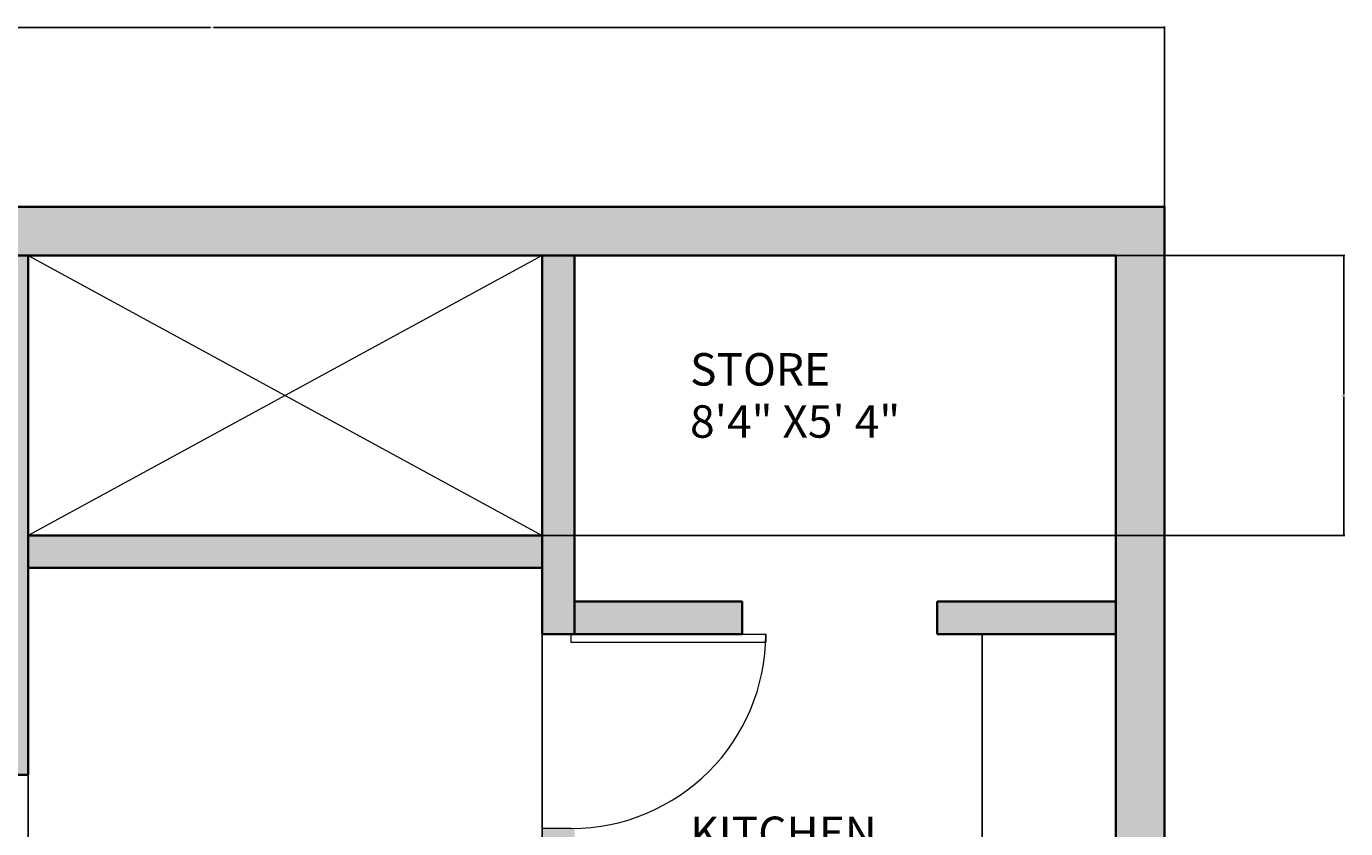
# Model space of a CAD drawing. Units: inches. Extents: x 2070 to 4408, y 1595 to 4269.
# Tile 18 of 20: x 2245 to 2489, y 2176 to 2325. Entities that reach past the tile are written whole.
import ezdxf

# ---------------------------------------------------------------- set-up
doc = ezdxf.new("R2010")
doc.units = ezdxf.units.IN
for name, color, linetype, lineweight in [('A-ANNO-DIMS', 2, 'Continuous', 18), ('A-AREA-IDEN', 7, 'Continuous', 18), ('A-DOOR', 4, 'Continuous', 18), ('A-FLOR-CASE', 8, 'Continuous', 18), ('A-FLOR-OPEN', 8, 'Continuous', 13), ('A-WALL', 7, 'Continuous', 35)]:
    doc.layers.add(name, color=color, linetype=linetype, lineweight=lineweight)
doc.layers.add('A-WALL-PATT', color=18, linetype='Continuous', lineweight=13, true_color=0x000000)
doc.styles.get("Standard").update_dxf_attribs({"font": 'arial.ttf'})
doc.dimstyles.get("Standard").update_dxf_attribs({"dimtxt": 0.18, "dimasz": 0.18, "dimexe": 0.18, "dimexo": 0.0625, "dimgap": 0.09, "dimtad": 0, "dimtih": 1, "dimtoh": 1, "dimdec": 4, "dimzin": 0, "dimdsep": 46, "dimtxsty": 'Standard', "dimcen": 0.09, "dimadec": 0, "dimazin": 0, "dimtfac": 1, "dimtdec": 4, "dimtofl": 0, "dimtmove": 0, "dimatfit": 3, "dimfxl": 1, "dimtolj": 1, "dimtzin": 0, "dimarcsym": 0})

# ---------------------------------------------------------------- blocks, each defined once
blk = doc.blocks.new('*U2')
for p, q in [((0, 0), (0, -6)), ((40, 0), (40, -6))]:
    blk.add_line(p, q)
blk.add_lwpolyline([(0, 0), (0, 40), (1.75, 40), (1.75, 0)], close=True)
blk.add_arc((0, 0), 40, 0, 90)
blk = doc.blocks.new('*D23')
at = {"layer": 'A-ANNO-DIMS', "color": 0, "lineweight": -2, "transparency": 16777216}
for p, q in [((2103.2, 2291.46), (2103.2, 2324.76)), ((2103.38, 2324.58), (2278.91, 2324.58)), ((2455.02, 2324.58), (2279.48, 2324.58)), ((2455.2, 2291.46), (2455.2, 2324.76))]:
    blk.add_line(p, q, dxfattribs=at)
at = {"layer": 'A-ANNO-DIMS', "color": 0, "transparency": 16777216}
for points in [[(2103.38, 2324.61), (2103.38, 2324.55), (2103.2, 2324.58)], [(2455.02, 2324.61), (2455.02, 2324.55), (2455.2, 2324.58)]]:
    blk.add_solid(points, dxfattribs=at)
at = {"layer": 'Defpoints', "color": 0, "transparency": 16777216}
for p in [(2455.2, 2324.58), (2103.2, 2291.4), (2455.2, 2291.4)]:
    blk.add_point(p, dxfattribs=at)
at = {"layer": 'A-ANNO-DIMS', "color": 0, "transparency": 16777216, "insert": (2279.2, 2324.58), "char_height": 0.18, "attachment_point": 5}
blk.add_mtext('\\A1;352', dxfattribs=at)
blk = doc.blocks.new('*D24')
at = {"layer": 'A-ANNO-DIMS', "color": 0, "lineweight": -2, "transparency": 16777216}
for p, q in [((2103.13, 2291.4), (2069.84, 2291.4)), ((2070.02, 2291.22), (2070.02, 1960.08)), ((2070.02, 1628.58), (2070.02, 1959.72)), ((2336.13, 1628.4), (2069.84, 1628.4))]:
    blk.add_line(p, q, dxfattribs=at)
at = {"layer": 'A-ANNO-DIMS', "color": 0, "transparency": 16777216}
for points in [[(2069.99, 2291.22), (2070.05, 2291.22), (2070.02, 2291.4)], [(2069.99, 1628.58), (2070.05, 1628.58), (2070.02, 1628.4)]]:
    blk.add_solid(points, dxfattribs=at)
at = {"layer": 'Defpoints', "color": 0, "transparency": 16777216}
for p in [(2070.02, 2291.4), (2103.2, 2291.4), (2336.2, 1628.4)]:
    blk.add_point(p, dxfattribs=at)
at = {"layer": 'A-ANNO-DIMS', "color": 0, "transparency": 16777216, "insert": (2070.02, 1959.9), "char_height": 0.18, "attachment_point": 5}
blk.add_mtext('\\A1;663', dxfattribs=at)
blk = doc.blocks.new('*D32')
at = {"layer": 'A-ANNO-DIMS', "color": 0, "lineweight": -2, "transparency": 16777216}
for p, q in [((2245.2, 2230.58), (2245.2, 1595.04)), ((2340.2, 2230.58), (2340.2, 1595.04)), ((2245.38, 1595.22), (2292.48, 1595.22)), ((2340.02, 1595.22), (2292.92, 1595.22))]:
    blk.add_line(p, q, dxfattribs=at)
at = {"layer": 'A-ANNO-DIMS', "color": 0, "transparency": 16777216}
for points in [[(2245.38, 1595.25), (2245.38, 1595.19), (2245.2, 1595.22)], [(2340.02, 1595.25), (2340.02, 1595.19), (2340.2, 1595.22)]]:
    blk.add_solid(points, dxfattribs=at)
at = {"layer": 'Defpoints', "color": 0, "transparency": 16777216}
for p in [(2245.2, 2230.65), (2340.2, 2230.65), (2340.2, 1595.22)]:
    blk.add_point(p, dxfattribs=at)
at = {"layer": 'A-ANNO-DIMS', "color": 0, "transparency": 16777216, "insert": (2292.7, 1595.22), "char_height": 0.18, "attachment_point": 5}
blk.add_mtext('\\A1;95', dxfattribs=at)
blk = doc.blocks.new('*D33')
at = {"layer": 'A-ANNO-DIMS', "color": 0, "lineweight": -2, "transparency": 16777216}
for p, q in [((2340.26, 2282.4), (2488.56, 2282.4)), ((2488.38, 2282.22), (2488.38, 2256.7)), ((2488.38, 2230.83), (2488.38, 2256.34)), ((2340.26, 2230.65), (2488.56, 2230.65))]:
    blk.add_line(p, q, dxfattribs=at)
at = {"layer": 'A-ANNO-DIMS', "color": 0, "transparency": 16777216}
for points in [[(2488.35, 2282.22), (2488.41, 2282.22), (2488.38, 2282.4)], [(2488.35, 2230.83), (2488.41, 2230.83), (2488.38, 2230.65)]]:
    blk.add_solid(points, dxfattribs=at)
at = {"layer": 'Defpoints', "color": 0, "transparency": 16777216}
for p in [(2340.2, 2282.4), (2488.38, 2282.4), (2340.2, 2230.65)]:
    blk.add_point(p, dxfattribs=at)
at = {"layer": 'A-ANNO-DIMS', "color": 0, "transparency": 16777216, "insert": (2488.38, 2256.52), "char_height": 0.18, "attachment_point": 5}
blk.add_mtext('\\A1;51.75', dxfattribs=at)
blk = doc.blocks.new('*D34')
at = {"layer": 'A-ANNO-DIMS', "color": 0, "lineweight": -2, "transparency": 16777216}
for p, q in [((2421.53, 2212.34), (2421.53, 1595.04)), ((2446.2, 2212.34), (2446.2, 1595.04)), ((2421.71, 1595.22), (2433.4, 1595.22)), ((2446.02, 1595.22), (2434.33, 1595.22))]:
    blk.add_line(p, q, dxfattribs=at)
at = {"layer": 'A-ANNO-DIMS', "color": 0, "transparency": 16777216}
for points in [[(2421.71, 1595.25), (2421.71, 1595.19), (2421.53, 1595.22)], [(2446.02, 1595.25), (2446.02, 1595.19), (2446.2, 1595.22)]]:
    blk.add_solid(points, dxfattribs=at)
at = {"layer": 'Defpoints', "color": 0, "transparency": 16777216}
for p in [(2421.53, 2212.4), (2446.2, 2212.4), (2446.2, 1595.22)]:
    blk.add_point(p, dxfattribs=at)
at = {"layer": 'A-ANNO-DIMS', "color": 0, "transparency": 16777216, "insert": (2433.86, 1595.22), "char_height": 0.18, "attachment_point": 5}
blk.add_mtext('\\A1;24.663', dxfattribs=at)

msp = doc.modelspace()

# ---------------------------------------------------------------- hatches: boundary and pattern name
at = {"layer": 'A-WALL-PATT'}
h = msp.add_hatch(color=256, dxfattribs=at)
h.dxf.hatch_style = 1
h.paths.add_polyline_path([(2346.196, 2218.3995), (2346.196, 2282.3995), (2340.196, 2282.3995), (2340.196, 2212.3995), (2345.5866, 2212.3995), (2346.196, 2212.3995)], flags=0)
h.paths.add_polyline_path([(2245.196, 2282.3995), (2239.196, 2282.3995), (2239.196, 2186.3995), (2244.5866, 2186.3995), (2245.196, 2186.3995)], flags=0)
h.paths.add_polyline_path([(2340.196, 2230.6455), (2245.196, 2230.6455), (2245.196, 2224.6455), (2340.196, 2224.6455)], flags=0)
h.paths.add_polyline_path([(2245.196, 2150.3995), (2239.196, 2150.3995), (2164.4362, 2150.3995), (2164.4362, 2144.3995), (2239.196, 2144.3995), (2239.196, 2086.3995), (2239.196, 2067.2711), (2244.5866, 2067.2711), (2245.196, 2067.2711), (2245.196, 2144.3995)], flags=0)
h.paths.add_polyline_path([(2346.196, 2176.3995), (2340.196, 2176.3995), (2340.196, 2086.3995), (2346.196, 2086.3995), (2346.196, 2125.318)], flags=0)
h.paths.add_polyline_path([(2446.196, 2086.3995), (2346.196, 2086.3995), (2340.196, 2086.3995), (2340.196, 2080.3995), (2446.196, 2080.3995)], flags=0)
h.paths.add_polyline_path([(2455.196, 2291.3995), (2103.196, 2291.3995), (2103.196, 1699.3995), (2336.196, 1699.3995), (2336.196, 1628.3995), (2345.196, 1628.3995), (2446.196, 1628.3995), (2454.8846, 1628.3995), (2454.8846, 1699.3995)])
h.paths.add_polyline_path([(2446.196, 2282.3995), (2446.196, 2218.3995), (2446.196, 2212.3995), (2446.196, 2086.3995), (2446.196, 2080.3995), (2446.196, 1708.3995), (2446.196, 1637.3995), (2345.196, 1637.3995), (2345.196, 1699.3995), (2345.196, 1708.3995), (2336.196, 1708.3995), (2112.196, 1708.3995), (2112.196, 2282.3995), (2239.196, 2282.3995), (2245.196, 2282.3995), (2356.196, 2282.3995)], flags=16)
h.paths.add_polyline_path([(2245.196, 2150.3995), (2245.196, 2144.3995), (2245.196, 2067.2711), (2244.5866, 2067.2711), (2239.196, 2067.2711), (2239.196, 2065.6988), (2203.2929, 2065.6988, 0.40145271), (2239.196, 2031.3337), (2244.5866, 2031.3337), (2245.196, 2031.2711), (2245.196, 1924.1525), (2239.196, 1924.1525), (2239.196, 1922.5803), (2203.2929, 1922.5803, 0.40145271), (2239.196, 1888.2151), (2244.5866, 1888.2151), (2245.196, 1888.1525), (2245.196, 1748.3995), (2339.196, 1748.4621, -0.40145271), (2303.2929, 1782.8272), (2303.2585, 1782.8272), (2303.2585, 1784.3995), (2339.196, 1784.3995), (2339.196, 1877.2067), (2291.196, 1877.2067), (2291.196, 1883.2067), (2291.196, 1946.3995), (2291.196, 1952.3995), (2291.196, 2086.3995), (2297.196, 2086.3995), (2302.196, 2086.3995), (2302.196, 2081.0259), (2303.7633, 2081.0259), (2303.7633, 2080.3995), (2338.0148, 2080.3995, 0.00437129), (2338.0203, 2081.0259), (2338.0203, 2086.3995), (2340.196, 2086.3995), (2340.196, 2176.4621), (2345.5866, 2176.4621, 0.40145271), (2381.4896, 2210.8272), (2345.5866, 2210.8272), (2345.5866, 2212.3995), (2340.196, 2212.3995), (2340.196, 2224.6455), (2245.196, 2224.6455), (2245.196, 2186.3995), (2244.5866, 2186.3995), (2239.196, 2186.3995), (2239.196, 2184.8272), (2203.2929, 2184.8272, 0.40145271), (2239.196, 2150.4621), (2244.5866, 2150.4621)], flags=0)
h.paths.add_polyline_path([(2346.196, 2282.3995), (2346.196, 2218.3995), (2377.1813, 2218.3995), (2377.1813, 2212.3995), (2346.196, 2212.3995), (2345.5866, 2212.3995), (2340.196, 2212.3995), (2340.196, 2224.6455), (2245.196, 2224.6455), (2245.196, 2230.6455), (2245.196, 2282.3995), (2292.696, 2256.5225), (2340.196, 2282.3995)], flags=0)
h.paths.add_polyline_path([(2346.196, 2086.3995), (2340.196, 2086.3995), (2340.196, 2080.3995), (2446.196, 2080.3995), (2431.196, 2016.3995), (2446.196, 1952.3995), (2412.196, 1952.3995), (2412.196, 2080.3995), (2340.196, 2080.3995), (2340.196, 2086.3995), (2340.196, 2176.3995), (2346.196, 2176.3995), (2346.196, 2125.318)], flags=0)
h.paths.add_polyline_path([(2186.508, 2270.0471, -0.03755288), (2186.9712, 2269.8581), (2186.9164, 2270.112, -0.02759121)], flags=0)
h.paths.add_polyline_path([(2183.955, 2273.7766, 1), (2188.2945, 2273.7766, 1)], flags=0)
h.paths.add_polyline_path([(2142.5261, 2274.6158, -0.03707541), (2142.5672, 2275.1696), (2142.5672, 2276.826), (2119.8759, 2276.826), (2119.8759, 2263.0962), (2140.4332, 2263.0962), (2142.5672, 2263.0962), (2142.5672, 2274.0621, -0.03707541)], flags=0)
h.paths.add_polyline_path([(2209.8974, 2263.0962), (2209.8974, 2262.2079), (2190.8042, 2262.2079), (2190.8042, 2263.0962)], flags=0)
h.paths.add_polyline_path([(2210.6382, 2276.1833), (2210.6382, 2263.9844), (2190.2185, 2263.9844), (2190.2185, 2276.1833)], flags=0)
h.paths.add_polyline_path([(2188.4362, 2273.7766, -1), (2183.8133, 2273.7766, -1)], flags=0)
h.paths.add_polyline_path([(2245.196, 2150.3995), (2245.196, 2144.3995), (2245.196, 2067.2711), (2239.196, 2067.2711), (2239.196, 2080.3995), (2172.196, 2080.3995), (2172.196, 2000.3995), (2239.196, 2000.3995), (2239.196, 1940.3995), (2159.0187, 1940.3995), (2123.0187, 1940.3995), (2112.196, 1940.3995), (2112.196, 1946.3995), (2123.0187, 1946.3995), (2123.0187, 1982.2238), (2124.586, 1982.2238), (2124.586, 1982.1895, -0.40145271), (2158.8429, 1946.3995), (2159.0187, 1946.3995), (2239.196, 1946.3995), (2239.196, 1994.3995), (2112.196, 1994.3995), (2112.196, 2000.3995), (2139.196, 2040.3995), (2112.196, 2080.3995), (2112.196, 2086.3995), (2239.196, 2086.3995), (2239.196, 2144.3995), (2209.5809, 2144.3995), (2209.5809, 2136.3995), (2203.0809, 2136.3995), (2205.0809, 2130.3996, -0.70257121), (2199.081, 2116.3995, -0.70256205), (2193.0809, 2130.3994), (2195.0809, 2136.3995), (2192.0809, 2136.3995), (2192.0809, 2134.8995), (2189.0809, 2134.8995), (2189.0809, 2135.8995), (2191.0809, 2135.8995), (2191.0809, 2136.3995), (2188.5809, 2136.3995), (2188.5809, 2144.3995), (2164.2481, 2144.3995, -0.39385849), (2130.0035, 2109.5491), (2130.0035, 2109.5147), (2128.4362, 2109.5147), (2128.4362, 2144.3995), (2112.196, 2144.3995), (2112.196, 2150.3995), (2128.4362, 2150.3995), (2128.4362, 2150.7127), (2164.4362, 2150.7127), (2164.4362, 2150.3995), (2239.196, 2150.3995)], flags=0)
h.paths.add_polyline_path([(2188.2075, 2266.8735), (2188.2075, 2211.8632, -0.41421356), (2185.4833, 2209.1391), (2146.7995, 2209.1391, -0.41421356), (2144.0754, 2211.8632), (2144.0754, 2266.8735, -0.41421356), (2146.7995, 2269.5976), (2185.4833, 2269.5976, -0.41421356)], flags=0)
h.paths.add_polyline_path([(2185.0844, 2273.7766, -1), (2187.1651, 2273.7766, -1)], flags=0)
h.paths.add_polyline_path([(2182.0486, 2259.2932), (2168.0953, 2259.2932), (2168.0953, 2260.8424), (2163.7261, 2260.8424), (2163.7261, 2259.2932), (2149.7727, 2259.2932), (2149.7727, 2266.3352), (2163.7261, 2266.3352), (2163.7261, 2261.9839), (2168.0953, 2261.9839), (2168.0953, 2266.3352), (2182.0486, 2266.3352)], flags=0)
h.paths.add_polyline_path([(2148.2585, 2250.2051), (2153.0615, 2241.8861, 0.39807048)], flags=0)
h.paths.add_polyline_path([(2162.7572, 2247.2885), (2153.1461, 2241.7396), (2148.1083, 2250.4653), (2157.7194, 2256.0142)], flags=0)
h.paths.add_polyline_path([(2162.6726, 2247.4351, -0.39286196), (2157.8415, 2255.6313), (2157.6431, 2255.6313), (2157.8696, 2255.7541)], flags=0)
h.paths.add_polyline_path([(2164.2604, 2145.339), (2164.4362, 2144.3995), (2164.4362, 2150.3995), (2164.2604, 2150.7127)], flags=0)
h.paths.add_polyline_path([(2208.5809, 2142.6495), (2208.5809, 2138.3995, -0.41421356), (2207.8309, 2137.3995), (2190.5809, 2137.3995, -0.41421356), (2189.5809, 2138.1495), (2189.5809, 2142.3995, -0.41421356), (2190.3309, 2143.3995), (2207.5809, 2143.3995, -0.41421356)], flags=0)
h.paths.add_polyline_path([(2147.957, 2229.9119), (2154.7494, 2223.1195, 0.39807048)], flags=0)
h.paths.add_polyline_path([(2162.7165, 2230.8473), (2154.8691, 2222.9998), (2147.7446, 2230.1244), (2155.592, 2237.9718)], flags=0)
h.paths.add_polyline_path([(2162.5969, 2230.9669, -0.39807048), (2155.8044, 2237.7594)], flags=0)
h.paths.add_polyline_path([(2391.8776, 2049.9192), (2408.5766, 2049.9192), (2408.5766, 2033.2202), (2408.5766, 1983.123), (2408.5766, 1966.4239), (2391.8776, 1966.4239), (2391.8776, 1983.123), (2341.7804, 1983.123), (2341.7804, 2033.2202), (2391.8776, 2033.2202)], flags=0)
h.paths.add_polyline_path([(2144.1055, 2274.6158, 1), (2148.445, 2274.6158, 1)], flags=0)
h.paths.add_polyline_path([(2148.5867, 2274.6158, -1), (2143.9638, 2274.6158, -1)], flags=0)
h.paths.add_polyline_path([(2145.2349, 2274.6158, -1), (2147.3156, 2274.6158, -1)], flags=0)
edge = h.paths.add_edge_path(flags=0)
edge.add_ellipse((2400.5951, 2040.9436), major_axis=(-4.5109, 0), ratio=0.97544784, start_angle=180, end_angle=270, ccw=False)
edge.add_ellipse((2400.5951, 2040.9436), major_axis=(-4.5109, 0), ratio=0.97544784, start_angle=90, end_angle=180, ccw=False)
edge.add_ellipse((2400.5951, 2040.9436), major_axis=(-4.5109, 0), ratio=0.97544784, start_angle=0, end_angle=90, ccw=False)
edge.add_ellipse((2400.5951, 2040.9436), major_axis=(-4.5109, 0), ratio=0.97544784, start_angle=270, end_angle=360, ccw=False)
h.paths.add_polyline_path([(2199.0809, 2117.3995, -0.73452973), (2195.0809, 2130.3995), (2203.081, 2130.3995, -0.73453329)], flags=0)
h.paths.add_polyline_path([(2141.9147, 2276.0353), (2141.9147, 2263.9844), (2120.4685, 2263.9844), (2120.4685, 2276.0353)], flags=0)
h.paths.add_polyline_path([(2138.4481, 2273.4072), (2138.4481, 2266.7226), (2133.2801, 2266.7226), (2133.2801, 2273.4072)], flags=0)
h.paths.add_polyline_path([(2137.9691, 2272.9175), (2137.9691, 2272.204), (2135.4229, 2272.204), (2135.4229, 2271.6329), (2135.3221, 2270.1051), (2135.3221, 2269.0265), (2135.4229, 2268.6811), (2135.4229, 2267.2011), (2133.7212, 2267.2011), (2133.7212, 2268.6811), (2133.7983, 2269.9587), (2133.7983, 2271.2758), (2133.7212, 2271.6329), (2133.7212, 2273.0065), (2135.717, 2273.0065), (2135.717, 2272.9175)], flags=0)
h.paths.add_polyline_path([(2137.9215, 2271.8264), (2137.9215, 2271.3786), (2137.5182, 2271.3786), (2136.9355, 2271.3786), (2136.3529, 2271.3786), (2135.7703, 2271.3786), (2135.7703, 2271.8264), (2136.1736, 2271.8264), (2136.7562, 2271.8264), (2137.3389, 2271.8264)], flags=0)
h.paths.add_polyline_path([(2137.9215, 2271.692), (2137.5182, 2271.692), (2136.9355, 2271.513), (2137.3389, 2271.513)], flags=0)
h.paths.add_polyline_path([(2136.3529, 2271.692), (2135.7703, 2271.513), (2136.1736, 2271.513), (2136.7562, 2271.692)], flags=0)
h.paths.add_polyline_path([(2137.9215, 2271.513), (2137.5182, 2271.513), (2136.7562, 2271.747), (2136.7562, 2271.692), (2137.3389, 2271.692)], flags=0)
h.paths.add_polyline_path([(2137.8207, 2270.4664), (2137.8207, 2270.0971), (2137.8207, 2269.627), (2137.8207, 2269.1569), (2137.8207, 2268.6868), (2137.3837, 2268.6868), (2136.6442, 2268.6868), (2135.9271, 2268.6868), (2135.9271, 2269.0562), (2135.9271, 2269.5263), (2135.9271, 2269.9963), (2135.9271, 2270.4664), (2136.3641, 2270.4664), (2137.0812, 2270.4664)], flags=0)
h.paths.add_polyline_path([(2137.3837, 2269.627), (2137.8207, 2269.627), (2137.8207, 2269.5263), (2137.3837, 2269.5263), (2137.3837, 2269.1569), (2137.8207, 2269.1569), (2137.3837, 2269.0562), (2137.3837, 2268.6868), (2137.0812, 2268.6868), (2137.0812, 2269.0562), (2136.6442, 2269.0562), (2136.6442, 2268.6868), (2136.3641, 2268.6868), (2136.3641, 2269.0562), (2135.9271, 2269.0562), (2135.9271, 2269.1569), (2136.3641, 2269.1569), (2136.3641, 2269.5263), (2135.9271, 2269.5263), (2135.9271, 2269.627), (2136.3641, 2269.627), (2136.3641, 2269.9963), (2135.9271, 2269.9963), (2136.3641, 2270.0971), (2136.3641, 2270.4664), (2136.6442, 2270.4664), (2136.6442, 2270.0971), (2137.0812, 2270.0971), (2137.0812, 2270.4664), (2137.3837, 2270.4664), (2137.3837, 2270.0971), (2137.8207, 2270.0971), (2137.3837, 2269.9963)], flags=0)
h.paths.add_polyline_path([(2137.5182, 2271.8264), (2137.5182, 2271.692), (2137.3389, 2271.3786), (2137.3389, 2271.513)], flags=0)
h.paths.add_polyline_path([(2137.8179, 2267.8138), (2137.8179, 2267.6879), (2137.1876, 2267.6879), (2136.4733, 2267.6879), (2135.759, 2267.6879), (2135.759, 2267.8138), (2136.3893, 2267.8138), (2137.1036, 2267.8138)], flags=0)
h.paths.add_polyline_path([(2137.0812, 2269.9963), (2137.0812, 2269.627), (2137.0812, 2269.1569), (2136.6442, 2269.1569), (2136.6442, 2269.5263), (2136.6442, 2269.9963)], flags=0)
h.paths.add_polyline_path([(2136.3529, 2271.8264), (2136.3529, 2271.692), (2136.1736, 2271.3786), (2136.1736, 2271.513)], flags=0)
h.paths.add_polyline_path([(2136.4733, 2267.8138), (2136.4733, 2267.6879), (2136.3893, 2267.6879), (2136.3893, 2267.8138)], flags=0)
h.paths.add_polyline_path([(2407.9087, 2032.5522), (2407.9087, 1983.7909), (2359.81, 1983.7909, -0.00912788), (2359.0575, 1983.7909), (2342.4483, 1983.7909), (2342.4483, 2032.5522)], flags=0)
h.paths.add_polyline_path([(2389.1838, 2023.1358), (2353.7856, 2023.1358), (2353.7856, 1985.4867, -0.09210376), (2350.2788, 1988.655), (2350.2788, 2026.6426), (2389.1838, 2026.6426)], flags=0)
h.paths.add_polyline_path([(2352.6166, 2024.3048), (2351.4477, 2024.3048), (2351.4477, 2025.4737), (2352.6166, 2025.4737)], flags=0)
h.paths.add_polyline_path([(2399.6319, 2026.7589), (2404.3661, 2026.7589, -0.41421356), (2407.0379, 2024.087), (2407.0379, 2013.4908, -0.41421356), (2404.3661, 2010.819), (2399.6319, 2010.819, -0.41421356), (2396.96, 2013.4908), (2396.96, 2024.087, -0.41421356)], flags=0)
h.paths.add_polyline_path([(2399.6319, 2026.0909), (2404.3661, 2026.0909, -0.41421356), (2406.37, 2024.087), (2406.37, 2013.4908, -0.41421356), (2404.3661, 2011.487), (2399.6319, 2011.487, -0.41421356), (2397.628, 2013.4908), (2397.628, 2024.087, -0.41421356)], flags=0)
h.paths.add_polyline_path([(2399.6319, 2002.3217), (2404.3661, 2002.3217, -0.41421356), (2407.0379, 1999.6498), (2407.0379, 1989.0536, -0.41421356), (2404.3661, 1986.3818), (2399.6319, 1986.3818, -0.41421356), (2396.96, 1989.0536), (2396.96, 1999.6498, -0.41421356)], flags=0)
h.paths.add_polyline_path([(2399.6319, 2001.6537), (2404.3661, 2001.6537, -0.41421356), (2406.37, 1999.6498), (2406.37, 1989.0536, -0.41421356), (2404.3661, 1987.0497), (2399.6319, 1987.0497, -0.41421356), (2397.628, 1989.0536), (2397.628, 1999.6498, -0.41421356)], flags=0)
edge = h.paths.add_edge_path(flags=0)
edge.add_ellipse((2400.5951, 1975.3996), major_axis=(-4.5109, 0), ratio=0.97544784, start_angle=-180, end_angle=-90, ccw=False)
edge.add_ellipse((2400.5951, 1975.3996), major_axis=(-4.5109, 0), ratio=0.97544784, start_angle=90, end_angle=180, ccw=False)
edge.add_ellipse((2400.5951, 1975.3996), major_axis=(-4.5109, 0), ratio=0.97544784, start_angle=0, end_angle=90, ccw=False)
edge.add_ellipse((2400.5951, 1975.3996), major_axis=(-4.5109, 0), ratio=0.97544784, start_angle=-90, end_angle=0, ccw=False)
h.paths.add_polyline_path([(2345.196, 1910.3995), (2366.4386, 1910.3995), (2366.4386, 1925.4555), (2392.3856, 1925.4555), (2392.3856, 1933.5025), (2400.1399, 1925.4555), (2392.3856, 1919.8795), (2392.3856, 1925.4555), (2366.4386, 1925.4555), (2366.4386, 1910.3995), (2381.196, 1910.3995), (2405.196, 1910.3995), (2405.196, 1898.3995), (2446.196, 1898.3995), (2446.196, 1886.3995), (2405.196, 1886.3995), (2405.196, 1874.3995), (2446.196, 1874.3995), (2446.196, 1862.3995), (2405.196, 1862.3995), (2405.196, 1850.3995), (2446.196, 1850.3995), (2446.196, 1838.3995), (2405.196, 1838.3995), (2405.196, 1826.3995), (2446.196, 1826.3995), (2446.196, 1814.3995), (2405.196, 1814.3995), (2405.196, 1802.3995), (2446.196, 1802.3995), (2446.196, 1798.3995), (2446.196, 1792.3995), (2405.196, 1792.3995), (2405.196, 1910.3995), (2381.196, 1910.3995), (2381.196, 1792.3995), (2345.196, 1792.3995)], flags=0)
h.paths.add_polyline_path([(2333.0944, 1863.3993, -0.41421356), (2334.7225, 1861.7712), (2334.7225, 1859.329), (2335.2653, 1859.329, -0.41421356), (2337.4361, 1857.1582), (2337.4361, 1843.862, -0.41421356), (2335.2653, 1841.6911, -0.41421356), (2337.4361, 1839.5203), (2337.4361, 1827.5808, -0.41421356), (2335.2653, 1825.41, -0.41421356), (2337.4361, 1823.2392), (2337.4361, 1808.5862, -0.41421356), (2335.2653, 1806.4153), (2334.7225, 1806.4153), (2334.7225, 1803.9732, -0.41421356), (2333.0944, 1802.3451), (2317.356, 1802.3451), (2317.0846, 1802.3451, -0.41421356), (2315.7279, 1803.7018), (2315.7279, 1803.8646), (2313.8284, 1803.8646, -0.41421356), (2311.6576, 1806.0354), (2311.6576, 1823.2015, -0.39597602), (2313.6834, 1825.3765, -0.43384798), (2311.6576, 1827.2718), (2311.6576, 1839.761, -0.41421356), (2313.5571, 1841.6604), (2313.8284, 1841.6604), (2333.8159, 1841.6604, -0.04213623), (2334.1798, 1841.6911, -0.41421356), (2332.009, 1843.862), (2332.009, 1857.1582, -0.41421356), (2334.1798, 1859.329), (2317.356, 1859.329), (2317.0846, 1859.329, -0.41421356), (2315.7279, 1860.6858), (2315.7279, 1862.0426, -0.41421356), (2317.0846, 1863.3993), (2317.356, 1863.3993)], flags=0)
h.paths.add_polyline_path([(2208.8475, 1848.9818), (2208.8475, 1840.9741, -0.41421356), (2207.0458, 1839.1724), (2206.5453, 1839.1721), (2206.5453, 1838.7218, -0.40985861), (2204.7704, 1836.9203), (2183.7501, 1836.9203, -0.41858196), (2181.9216, 1838.7218), (2181.9216, 1839.1721), (2181.421, 1839.1724, -0.41421356), (2179.6193, 1840.9741), (2179.6193, 1848.6817, -0.44064415), (2185.1126, 1854.9874), (2203.3852, 1854.9874, -0.45707961)], flags=0)
h.paths.add_polyline_path([(2204.243, 1848.4815), (2204.243, 1848.4815, 0.41725335), (2202.2204, 1850.4833), (2186.2049, 1850.4833, 0.4111805), (2184.2237, 1848.4815), (2184.2237, 1848.4815, -0.4111807), (2186.2049, 1850.4833), (2202.2204, 1850.4833, -0.41725315)], flags=0)
h.paths.add_polyline_path([(2234.7177, 1830.228), (2234.7176, 1781.6047, -0.41421356), (2233.4381, 1780.3252), (2218.6064, 1780.3252, -0.41421356), (2217.8387, 1781.0929), (2217.8387, 1783.3961, -0.41421356), (2218.6064, 1784.1639), (2218.6065, 1796.9595, -0.41421356), (2219.886, 1798.239, -0.41421356), (2218.6065, 1799.5186), (2218.6065, 1812.3142, -0.41421356), (2219.8861, 1813.5938, -0.41421356), (2218.6065, 1814.8733), (2218.6065, 1827.6689, -0.41421356), (2217.8388, 1828.4367), (2217.8388, 1830.7399, -0.41421356), (2218.6065, 1831.5076), (2233.4382, 1831.5076, -0.41421356)], flags=0)
h.paths.add_polyline_path([(2230.6344, 1827.6689, -0.41421356), (2231.4021, 1826.9012), (2231.4021, 1784.9316, -0.41421356), (2230.6343, 1784.1639), (2221.1853, 1784.1639), (2221.1853, 1827.6689)], flags=0)
h.paths.add_polyline_path([(2222.7208, 1798.239), (2221.6971, 1798.239), (2221.6971, 1813.5938), (2222.7208, 1813.5938)], flags=0)
h.paths.add_polyline_path([(2206.5453, 1773.935), (2206.5453, 1773.4848), (2206.9457, 1773.4848), (2207.0458, 1773.4845, -0.41421356), (2208.8475, 1771.6827), (2208.8475, 1763.675, -0.44222432), (2203.6505, 1757.6695), (2185.3851, 1757.6695, -0.45508402), (2179.6193, 1763.9752), (2179.6193, 1771.6827, -0.41421356), (2181.421, 1773.4845), (2181.421, 1773.4848), (2181.9216, 1773.4848), (2181.9216, 1773.935, -0.40985861), (2183.6965, 1775.7366), (2204.7167, 1775.7366, -0.41858196)], flags=0)
h.paths.add_polyline_path([(2202.2619, 1762.1736), (2186.2464, 1762.1736, -0.41725315), (2184.2237, 1764.1754), (2184.2237, 1764.1754, 0.41725335), (2186.2464, 1762.1736), (2202.2619, 1762.1736, 0.4111805), (2204.243, 1764.1754), (2204.243, 1764.1754, -0.4111807)], flags=0)
h.paths.add_polyline_path([(2313.0034, 1713.1906), (2312.997, 1713.1697), (2313.0123, 1713.1612)], flags=0)
h.paths.add_polyline_path([(2305.7314, 1721.0488), (2305.6257, 1721.1994), (2305.4853, 1721.084)], flags=0)
h.paths.add_polyline_path([(2307.5562, 1726.1427), (2307.6186, 1726.1026), (2307.5737, 1726.0477), (2308.5692, 1720.6434), (2310.5345, 1721.2985), (2310.5721, 1721.411), (2310.6958, 1721.3523), (2313.8453, 1722.4021), (2314.9351, 1723.8033), (2314.9294, 1723.9165), (2315.0028, 1723.8903), (2313.874, 1722.4389), (2313.8697, 1722.4102), (2308.5692, 1720.6434), (2308.9864, 1720.122), (2309.0665, 1720.0971), (2309.053, 1720.0387), (2310.9235, 1717.7005), (2311.4182, 1717.6259), (2311.2918, 1717.2402), (2312.0655, 1716.2731), (2312.1081, 1716.2606), (2312.0969, 1716.2339), (2308.5692, 1720.6434), (2305.2249, 1717.745), (2305.232, 1717.704), (2305.1665, 1717.6944), (2308.5692, 1720.6434)], flags=0)
h.paths.add_polyline_path([(2288.2072, 1714.3431), (2288.2008, 1714.3222), (2288.216, 1714.3137)], flags=0)
h.paths.add_polyline_path([(2280.9352, 1722.2013), (2280.8295, 1722.3519), (2280.689, 1722.2365)], flags=0)
h.paths.add_polyline_path([(2282.76, 1727.2952), (2282.8224, 1727.2551), (2282.7775, 1727.2002), (2283.773, 1721.7959), (2285.7383, 1722.451), (2285.7759, 1722.5635), (2285.8995, 1722.5048), (2289.0491, 1723.5546), (2290.1389, 1724.9558), (2290.1332, 1725.069), (2290.2065, 1725.0428), (2289.0777, 1723.5915), (2289.0735, 1723.5628), (2283.773, 1721.7959), (2284.1901, 1721.2745), (2284.2703, 1721.2496), (2284.2567, 1721.1913), (2286.1273, 1718.8531), (2286.622, 1718.7785), (2286.4956, 1718.3927), (2287.2692, 1717.4256), (2287.3119, 1717.4131), (2287.3006, 1717.3864), (2283.773, 1721.7959), (2280.4286, 1718.8975), (2280.4357, 1718.8565), (2280.3703, 1718.8469), (2283.773, 1721.7959)], flags=0)
h.paths.add_polyline_path([(2302.0672, 1721.8694), (2301.8205, 1721.8572), (2301.7578, 1722.1787), (2299.415, 1724.5215), (2299.103, 1724.4694), (2299.0662, 1724.8703)], flags=0)
h.paths.add_polyline_path([(2264.5643, 1715.4956), (2264.5579, 1715.4747), (2264.5731, 1715.4662)], flags=0)
h.paths.add_polyline_path([(2257.2923, 1723.3538), (2257.1865, 1723.5044), (2257.0461, 1723.389)], flags=0)
h.paths.add_polyline_path([(2259.117, 1728.4477), (2259.1795, 1728.4077), (2259.1345, 1728.3527), (2260.13, 1722.9484), (2262.0954, 1723.6036), (2262.133, 1723.716), (2262.2566, 1723.6573), (2265.4061, 1724.7071), (2266.4959, 1726.1083), (2266.4902, 1726.2215), (2266.5636, 1726.1953), (2265.4348, 1724.744), (2265.4305, 1724.7153), (2260.13, 1722.9484), (2260.5472, 1722.427), (2260.6273, 1722.4022), (2260.6138, 1722.3438), (2262.4843, 1720.0056), (2262.979, 1719.931), (2262.8526, 1719.5452), (2263.6263, 1718.5781), (2263.6689, 1718.5656), (2263.6577, 1718.5389), (2260.13, 1722.9484), (2256.7857, 1720.05), (2256.7928, 1720.009), (2256.7273, 1719.9994), (2260.13, 1722.9484)], flags=0)
h.paths.add_polyline_path([(2277.2709, 1723.0219), (2277.0243, 1723.0097), (2276.9616, 1723.3312), (2274.6187, 1725.6741), (2274.3067, 1725.6219), (2274.27, 1726.0228)], flags=0)
h.paths.add_polyline_path([(2253.628, 1724.1744), (2253.3814, 1724.1622), (2253.3186, 1724.4838), (2250.9758, 1726.8266), (2250.6638, 1726.7744), (2250.627, 1727.1753)], flags=0)
h.paths.add_polyline_path([(2161.9194, 1715.4956), (2161.913, 1715.4747), (2161.9282, 1715.4662)], flags=0)
h.paths.add_polyline_path([(2154.6474, 1723.3538), (2154.5416, 1723.5044), (2154.4012, 1723.389)], flags=0)
h.paths.add_polyline_path([(2162.7899, 1724.744), (2162.7856, 1724.7153), (2157.4851, 1722.9484), (2157.9023, 1722.427), (2157.9824, 1722.4022), (2157.9689, 1722.3438), (2159.8394, 1720.0056), (2160.3341, 1719.931), (2160.2078, 1719.5452), (2160.9814, 1718.5781), (2161.024, 1718.5656), (2161.0128, 1718.5389), (2157.4851, 1722.9484), (2154.1408, 1720.05), (2154.1479, 1720.009), (2154.0824, 1719.9994), (2157.4851, 1722.9484), (2156.4721, 1728.4477), (2156.5346, 1728.4077), (2156.4896, 1728.3527), (2157.4851, 1722.9484), (2159.4505, 1723.6036), (2159.4881, 1723.716), (2159.6117, 1723.6573), (2162.7612, 1724.7071), (2163.851, 1726.1083), (2163.8453, 1726.2215), (2163.9187, 1726.1953)], flags=0)
h.paths.add_polyline_path([(2150.9831, 1724.1744), (2150.7365, 1724.1622), (2150.6738, 1724.4838), (2148.3309, 1726.8266), (2148.0189, 1726.7744), (2147.9822, 1727.1753)], flags=0)
h.paths.add_polyline_path([(2132.5099, 1716.6482), (2132.5035, 1716.6272), (2132.5187, 1716.6187)], flags=0)
h.paths.add_polyline_path([(2125.2379, 1724.5064), (2125.1322, 1724.6569), (2124.9917, 1724.5415)], flags=0)
h.paths.add_polyline_path([(2133.3804, 1725.8965), (2133.3762, 1725.8678), (2128.0757, 1724.101), (2128.4928, 1723.5795), (2128.5729, 1723.5547), (2128.5594, 1723.4963), (2130.43, 1721.1581), (2130.9246, 1721.0835), (2130.7983, 1720.6977), (2131.5719, 1719.7306), (2131.6146, 1719.7181), (2131.6033, 1719.6914), (2128.0757, 1724.101), (2124.7313, 1721.2025), (2124.7384, 1721.1615), (2124.6729, 1721.1519), (2128.0757, 1724.101), (2127.0626, 1729.6002), (2127.1251, 1729.5602), (2127.0801, 1729.5052), (2128.0757, 1724.101), (2130.041, 1724.7561), (2130.0786, 1724.8685), (2130.2022, 1724.8098), (2133.3517, 1725.8597), (2134.4415, 1727.2608), (2134.4358, 1727.3741), (2134.5092, 1727.3478)], flags=0)
h.paths.add_polyline_path([(2121.5736, 1725.3269), (2121.327, 1725.3148), (2121.2643, 1725.6363), (2118.9214, 1727.9791), (2118.6094, 1727.9269), (2118.5727, 1728.3279)], flags=0)
h.paths.add_polyline_path([(2433.3904, 1646.406), (2433.384, 1646.3851), (2433.3992, 1646.3766)], flags=0)
h.paths.add_polyline_path([(2426.1184, 1654.2642), (2426.0127, 1654.4148), (2425.8722, 1654.2994)], flags=0)
h.paths.add_polyline_path([(2427.9432, 1659.3581), (2428.0056, 1659.318), (2427.9606, 1659.2631), (2428.9562, 1653.8588), (2430.9215, 1654.514), (2430.9591, 1654.6264), (2431.0827, 1654.5677), (2434.2323, 1655.6175), (2435.322, 1657.0187), (2435.3163, 1657.1319), (2435.3897, 1657.1057), (2434.2609, 1655.6544), (2434.2567, 1655.6257), (2428.9562, 1653.8588), (2429.3733, 1653.3374), (2429.4534, 1653.3126), (2429.4399, 1653.2542), (2431.3105, 1650.916), (2431.8051, 1650.8414), (2431.6788, 1650.4556), (2432.4524, 1649.4885), (2432.4951, 1649.476), (2432.4838, 1649.4493), (2428.9562, 1653.8588), (2425.6118, 1650.9604), (2425.6189, 1650.9194), (2425.5535, 1650.9098), (2428.9562, 1653.8588)], flags=0)
h.paths.add_polyline_path([(2376.63, 1645.4912), (2376.6236, 1645.4703), (2376.6388, 1645.4617)], flags=0)
h.paths.add_polyline_path([(2369.358, 1653.3494), (2369.2523, 1653.5), (2369.1118, 1653.3845)], flags=0)
h.paths.add_polyline_path([(2371.1828, 1658.4432), (2371.2452, 1658.4032), (2371.2003, 1658.3482), (2372.1958, 1652.944), (2374.1611, 1653.5991), (2374.1987, 1653.7116), (2374.3224, 1653.6528), (2377.4719, 1654.7027), (2378.5617, 1656.1038), (2378.556, 1656.2171), (2378.6293, 1656.1908), (2377.5005, 1654.7395), (2377.4963, 1654.7108), (2372.1958, 1652.944), (2372.6129, 1652.4225), (2372.6931, 1652.3977), (2372.6795, 1652.3393), (2374.5501, 1650.0011), (2375.0448, 1649.9265), (2374.9184, 1649.5407), (2375.692, 1648.5737), (2375.7347, 1648.5611), (2375.7234, 1648.5344), (2372.1958, 1652.944), (2368.8514, 1650.0456), (2368.8586, 1650.0046), (2368.7931, 1649.995), (2372.1958, 1652.944)], flags=0)
h.paths.add_polyline_path([(2404.0947, 1645.0338), (2404.0883, 1645.0128), (2404.1035, 1645.0043)], flags=0)
h.paths.add_polyline_path([(2396.8227, 1652.892), (2396.717, 1653.0425), (2396.5765, 1652.9271)], flags=0)
h.paths.add_polyline_path([(2398.6475, 1657.9858), (2398.7099, 1657.9458), (2398.665, 1657.8908), (2399.6605, 1652.4866), (2401.6258, 1653.1417), (2401.6634, 1653.2541), (2401.7871, 1653.1954), (2404.9366, 1654.2453), (2406.0264, 1655.6464), (2406.0207, 1655.7596), (2406.094, 1655.7334), (2404.9652, 1654.2821), (2404.961, 1654.2534), (2399.6605, 1652.4866), (2400.0776, 1651.9651), (2400.1578, 1651.9403), (2400.1442, 1651.8819), (2402.0148, 1649.5437), (2402.5095, 1649.4691), (2402.3831, 1649.0833), (2403.1567, 1648.1162), (2403.1994, 1648.1037), (2403.1881, 1648.077), (2399.6605, 1652.4866), (2396.3162, 1649.5881), (2396.3233, 1649.5471), (2396.2578, 1649.5375), (2399.6605, 1652.4866)], flags=0)
h.paths.add_polyline_path([(2419.4532, 1658.0857), (2422.4541, 1655.0848), (2422.2075, 1655.0726), (2422.1448, 1655.3941), (2419.8019, 1657.737), (2419.4899, 1657.6848)], flags=0)
h.paths.add_polyline_path([(2390.1575, 1656.7135), (2393.1584, 1653.7125), (2392.9118, 1653.7004), (2392.8491, 1654.0219), (2390.5063, 1656.3647), (2390.1943, 1656.3125)], flags=0)
h.paths.add_polyline_path([(2362.6928, 1657.1709), (2365.6937, 1654.1699), (2365.4471, 1654.1578), (2365.3844, 1654.4793), (2363.0416, 1656.8221), (2362.7295, 1656.77)], flags=0)
h.paths.add_polyline_path([(2419.9523, 2037.8601), (2440.2872, 2037.8601), (2440.2872, 2047.1732), (2419.9523, 2047.1732)], flags=8)
h.paths.add_polyline_path([(2370.186, 1698.9005), (2413.6287, 1698.9005), (2413.6287, 1708.0908), (2370.186, 1708.0908)], flags=8)
h.paths.add_polyline_path([(2370.1656, 1708.5185), (2430.0857, 1708.5185), (2430.0857, 1717.8316), (2370.1656, 1717.8316)], flags=8)
h.paths.add_polyline_path([(2254.1469, 1788.1883), (2302.2471, 1788.1883), (2302.2471, 1797.3786), (2254.1469, 1797.3786)], flags=8)
h.paths.add_polyline_path([(2254.1264, 1797.8063), (2326.1448, 1797.8063), (2326.1448, 1807.1194), (2254.1264, 1807.1194)], flags=8)
h.paths.add_polyline_path([(2300.08, 1914.5069), (2338.861, 1914.5069), (2338.861, 1923.6972), (2300.08, 1923.6972)], flags=8)
h.paths.add_polyline_path([(2300.0595, 1924.1249), (2331.5882, 1924.1249), (2331.5882, 1933.438), (2300.0595, 1933.438)], flags=8)
h.paths.add_polyline_path([(2176.6905, 1716.4567), (2224.1441, 1716.4567), (2224.1441, 1725.647), (2176.6905, 1725.647)], flags=8)
h.paths.add_polyline_path([(2176.67, 1726.0747), (2245.9176, 1726.0747), (2245.9176, 1735.3878), (2176.67, 1735.3878)], flags=8)
h.paths.add_polyline_path([(2339.997, 2039.7696), (2388.1034, 2039.7696), (2388.1034, 2048.9661), (2339.997, 2048.9661)], flags=8)
h.paths.add_polyline_path([(2339.9776, 2049.3928), (2388.7204, 2049.3928), (2388.7204, 2058.7059), (2339.9776, 2058.7059)], flags=8)
h.paths.add_polyline_path([(2366.0063, 2161.3825), (2409.449, 2161.3825), (2409.449, 2170.5728), (2366.0063, 2170.5728)], flags=8)
h.paths.add_polyline_path([(2365.9868, 2171.0016), (2405.879, 2171.0016), (2405.879, 2180.3085), (2365.9868, 2180.3085)], flags=8)
h.paths.add_polyline_path([(2366.0102, 2247.0726), (2407.12, 2247.0726), (2407.12, 2256.263), (2366.0102, 2256.263)], flags=8)
h.paths.add_polyline_path([(2365.9897, 2256.6906), (2397.9686, 2256.6906), (2397.9686, 2266.0037), (2365.9897, 2266.0037)], flags=8)
h.paths.add_polyline_path([(2271.8465, 2102.7885), (2307.6541, 2102.7885), (2307.6541, 2111.9849), (2271.8465, 2111.9849)], flags=8)
h.paths.add_polyline_path([(2271.8281, 2112.4126), (2304.2673, 2112.4126), (2304.2673, 2121.7196), (2271.8281, 2121.7196)], flags=8)
h.paths.add_polyline_path([(2141.6408, 2187.5934), (2182.108, 2187.5934), (2182.108, 2196.7837), (2141.6408, 2196.7837)], flags=8)
h.paths.add_polyline_path([(2141.6203, 2197.2114), (2190.3631, 2197.2114), (2190.3631, 2206.5245), (2141.6203, 2206.5245)], flags=8)
h.paths.add_polyline_path([(2165.7271, 2103.039), (2211.5027, 2103.039), (2211.5027, 2112.2293), (2165.7271, 2112.2293)], flags=8)
h.paths.add_polyline_path([(2165.7077, 2112.658), (2185.1033, 2112.658), (2185.1033, 2121.965), (2165.7077, 2121.965)], flags=8)
h.paths.add_polyline_path([(2174.945, 2048.0789), (2211.3973, 2048.0789), (2211.3973, 2057.2693), (2174.945, 2057.2693)], flags=8)
h.paths.add_polyline_path([(2174.9256, 2057.698), (2194.3212, 2057.698), (2194.3212, 2067.0049), (2174.9256, 2067.0049)], flags=8)
h.paths.add_polyline_path([(2164.8305, 1965.8394), (2202.9649, 1965.8394), (2202.9649, 1975.0297), (2164.8305, 1975.0297)], flags=8)
h.paths.add_polyline_path([(2164.8111, 1975.4584), (2184.2067, 1975.4584), (2184.2067, 1984.7654), (2164.8111, 1984.7654)], flags=8)
h.paths.add_polyline_path([(2133.0392, 1862.086), (2173.5065, 1862.086), (2173.5065, 1871.2763), (2133.0392, 1871.2763)], flags=8)
h.paths.add_polyline_path([(2133.0709, 1871.8585), (2157.0382, 1871.8585), (2157.0382, 1880.8585), (2133.0709, 1880.8585)], flags=8)
h.paths.add_polyline_path([(2406.4423, 1923.5541), (2418.8209, 1923.5541), (2418.8209, 1932.7199), (2406.4423, 1932.7199)], flags=8)
h = msp.add_hatch(color=256, dxfattribs=at)
h.dxf.hatch_style = 1
h.paths.add_polyline_path([(2245.196, 2282.3995), (2239.196, 2282.3995), (2239.196, 2186.3995), (2244.5866, 2186.3995), (2245.196, 2186.3995)])
h.paths.add_polyline_path([(2340.196, 2230.6455), (2245.196, 2230.6455), (2245.196, 2224.6455), (2340.196, 2224.6455)])
h.paths.add_polyline_path([(2346.196, 2282.3995), (2340.196, 2282.3995), (2340.196, 2212.3995), (2345.5866, 2212.3995), (2346.196, 2212.3995), (2346.196, 2218.3995)])
h.paths.add_polyline_path([(2245.196, 2144.3995), (2245.196, 2150.3995), (2239.196, 2150.3995), (2164.4362, 2150.3995), (2164.4362, 2144.3995), (2239.196, 2144.3995), (2239.196, 2086.3995), (2239.196, 2067.2711), (2244.5866, 2067.2711), (2245.196, 2067.2711)])
h.paths.add_polyline_path([(2128.4362, 2150.3995), (2112.196, 2150.3995), (2112.196, 2144.3995), (2128.4362, 2144.3995), (2128.4362, 2145.339)])
h.paths.add_polyline_path([(2239.196, 2086.3995), (2112.196, 2086.3995), (2112.196, 2080.3995), (2239.196, 2080.3995)])
h.paths.add_polyline_path([(2172.196, 2080.3995), (2166.196, 2080.3995), (2166.196, 2000.3995), (2172.196, 2000.3995)])
h.paths.add_polyline_path([(2239.196, 2000.3995), (2112.196, 2000.3995), (2112.196, 1994.3995), (2239.196, 1994.3995)])
h.paths.add_polyline_path([(2245.196, 2031.2711), (2239.196, 2031.2711), (2239.196, 2000.3995), (2239.196, 1940.3995), (2245.196, 1940.3995)])
h.paths.add_polyline_path([(2239.196, 1946.3995), (2159.0187, 1946.3995), (2159.0187, 1940.3995), (2239.196, 1940.3995)])
h.paths.add_polyline_path([(2123.0187, 1946.3995), (2112.196, 1946.3995), (2112.196, 1940.3995), (2123.0187, 1940.3995)])
h.paths.add_polyline_path([(2377.1813, 2218.3995), (2346.196, 2218.3995), (2346.196, 2212.3995), (2377.1813, 2212.3995)])
h.paths.add_polyline_path([(2446.196, 2218.3995), (2413.1813, 2218.3995), (2413.1813, 2212.3995), (2446.196, 2212.3995)])
h.paths.add_polyline_path([(2446.196, 2086.3995), (2346.196, 2086.3995), (2340.196, 2086.3995), (2340.196, 2080.3995), (2446.196, 2080.3995)], flags=17)
h.paths.add_polyline_path([(2346.196, 2125.318), (2346.196, 2176.3995), (2340.196, 2176.3995), (2340.196, 2086.3995), (2346.196, 2086.3995)])
h.paths.add_polyline_path([(2245.196, 1888.1525), (2239.196, 1888.1525), (2239.196, 1748.3995), (2245.196, 1748.3995)])
h.paths.add_polyline_path([(2345.196, 1748.3995), (2239.196, 1748.3995), (2112.196, 1748.3995), (2112.196, 1742.3995), (2239.196, 1742.3995), (2345.196, 1742.3995)])
h.paths.add_polyline_path([(2297.196, 2080.3995), (2297.196, 2086.3995), (2291.196, 2086.3995), (2291.196, 1952.3995), (2291.196, 1946.3995), (2339.196, 1946.3995), (2339.196, 1883.2067), (2291.196, 1883.2067), (2291.196, 1877.2067), (2339.196, 1877.2067), (2339.196, 1784.3995), (2345.196, 1784.3995), (2345.196, 1792.3995), (2345.196, 1946.3995), (2446.196, 1946.3995), (2446.196, 1952.3995), (2297.196, 1952.3995)])

# ---------------------------------------------------------------- linework, layer by layer
at = {"layer": 'A-FLOR-CASE'}
for p, q in [((2446.196, 2212.3995), (2421.5333, 2212.3995)), ((2421.5333, 2212.3995), (2421.5333, 2122.3995))]:
    msp.add_line(p, q, dxfattribs=at)
at = {"layer": 'A-FLOR-OPEN'}
for p, q in [((2245.196, 2282.3995), (2340.196, 2230.6455)), ((2340.196, 2282.3995), (2245.196, 2230.6455))]:
    msp.add_line(p, q, dxfattribs=at)
at = {"layer": 'A-WALL'}
for p, q in [((2245.196, 2186.3995), (2245.196, 2282.3995)), ((2245.196, 2282.3995), (2356.196, 2282.3995)), ((2245.196, 2282.3995), (2245.196, 2224.6455)), ((2346.196, 2282.3995), (2340.196, 2282.3995)), ((2340.196, 2282.3995), (2340.196, 2212.3995)), ((2340.196, 2282.3995), (2340.196, 2282.3995)), ((2446.196, 2282.3995), (2346.196, 2282.3995)), ((2346.196, 2282.3995), (2346.196, 2218.3995)), ((2446.196, 2282.3995), (2446.196, 2218.3995)), ((2340.196, 2230.6455), (2245.196, 2230.6455)), ((2340.196, 2224.6455), (2340.196, 2230.6455)), ((2340.196, 2230.6455), (2340.196, 2224.6455)), ((2245.196, 2224.6455), (2340.196, 2224.6455)), ((2346.196, 2218.3995), (2346.196, 2212.3995)), ((2377.1813, 2218.3995), (2346.196, 2218.3995)), ((2377.1813, 2212.3995), (2377.1813, 2218.3995)), ((2446.196, 2218.3995), (2413.1813, 2218.3995)), ((2413.1813, 2212.3995), (2413.1813, 2218.3995)), ((2446.196, 2218.3995), (2446.196, 2212.3995)), ((2346.196, 2212.3995), (2340.196, 2212.3995)), ((2346.196, 2212.3995), (2377.1813, 2212.3995)), ((2346.196, 2212.3995), (2377.1813, 2212.3995)), ((2413.1813, 2212.3995), (2446.196, 2212.3995)), ((2446.196, 2212.3995), (2446.196, 2086.3995)), ((2245.196, 2186.3995), (2239.196, 2186.3995))]:
    msp.add_line(p, q, dxfattribs=at)
for points in [[(2336.196, 1699.3995), (2103.196, 1699.3995), (2103.196, 2291.3995), (2455.196, 2291.3995), (2455.196, 1699.3995), (2454.8846, 1699.3995)], [(2336.196, 1708.3995), (2112.196, 1708.3995), (2112.196, 2282.3995), (2446.196, 2282.3995), (2446.196, 2218.3995)], [(2446.196, 2212.3995), (2446.196, 1708.3995)]]:
    msp.add_lwpolyline(points, dxfattribs=at)

# ---------------------------------------------------------------- block references
at = {"layer": 'A-DOOR', "xscale": 0.8984361948159364, "yscale": 0.8984361948159364, "zscale": 0.8984361948159364, "rotation": 270}
msp.add_blockref('*U2', (2345.5866, 2212.3995), dxfattribs=at)

# ---------------------------------------------------------------- texts
at = {"layer": 'A-AREA-IDEN'}
for s, p in [('STORE', (2367.5419, 2258.3452)), ('8\'4" X5\' 4"', (2367.5419, 2248.7067)), ('KITCHEN', (2367.538, 2172.655))]:
    msp.add_text(s, height=6, dxfattribs=at).set_placement(p)

# ---------------------------------------------------------------- dimensions: what is measured, and where the dimension line sits
at = {"layer": 'A-ANNO-DIMS'}
for base, p1, p2, override, picture, middle in [((2455.196, 2324.5795), (2103.196, 2291.3995), (2455.196, 2291.3995), {"dimdec": 0, "dimlfac": 1, "dimrnd": 0, "dimzin": 0, "dimdsep": 46, "dimlunit": 2}, '*D23', (2279.196, 2324.5795)), ((2340.196, 1595.2195), (2245.196, 2230.6455), (2340.196, 2230.6455), {"dimdec": 0, "dimlfac": 1, "dimrnd": 0, "dimzin": 0, "dimdsep": 46, "dimlunit": 2}, '*D32', (2292.696, 1595.2195)), ((2446.196, 1595.2195), (2421.5333, 2212.3995), (2446.196, 2212.3995), {"dimdec": 3, "dimlfac": 1, "dimrnd": 0, "dimzin": 0, "dimdsep": 46, "dimlunit": 2}, '*D34', (2433.8646, 1595.2195))]:
    dim = msp.add_linear_dim(base=base, p1=p1, p2=p2, dimstyle='Standard', override=override, dxfattribs=at)
    dim.commit()
    dim.dimension.update_dxf_attribs({"geometry": picture, "text_midpoint": middle})
for base, p1, p2, override, picture, middle in [((2070.016, 2291.3995), (2336.196, 1628.3995), (2103.196, 2291.3995), {"dimdec": 0, "dimlfac": 1, "dimrnd": 0, "dimzin": 0, "dimdsep": 46, "dimlunit": 2}, '*D24', (2070.016, 1959.8995)), ((2488.376, 2282.3995), (2340.196, 2230.6455), (2340.196, 2282.3995), {"dimdec": 2, "dimlfac": 1, "dimrnd": 0, "dimzin": 0, "dimdsep": 46, "dimlunit": 2}, '*D33', (2488.376, 2256.5225))]:
    dim = msp.add_linear_dim(base=base, p1=p1, p2=p2, angle=90, dimstyle='Standard', override=override, dxfattribs=at)
    dim.commit()
    dim.dimension.update_dxf_attribs({"geometry": picture, "text_midpoint": middle})

doc.saveas('drawing.dxf')
